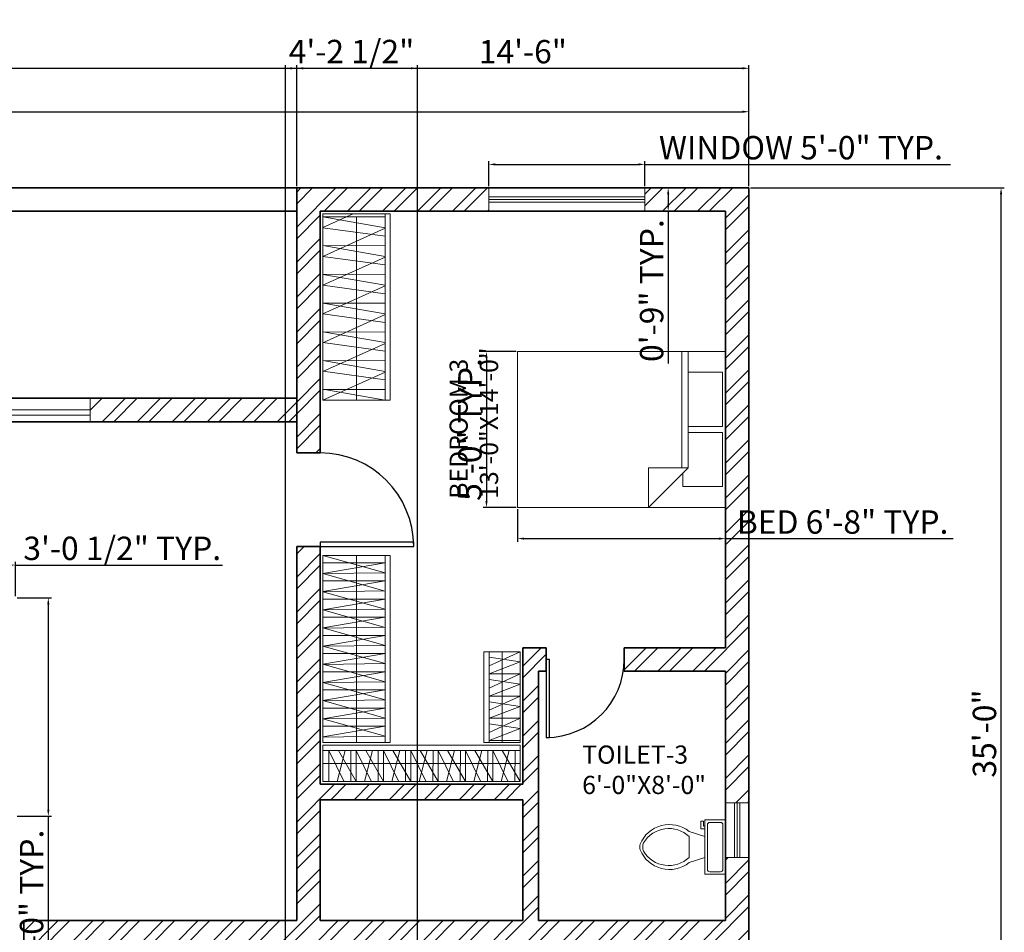
# Model space of a CAD drawing. Units: inches. Extents: x 416 to 1422, y 799 to 1634.
# Tile 5 of 5: x 1043 to 1422, y 1283 to 1634. Entities that reach past the tile are written whole.
import ezdxf

# ---------------------------------------------------------------- set-up
doc = ezdxf.new("R2010")
doc.units = ezdxf.units.IN
for name, color, linetype, lineweight in [('A-ANNO-DIMS', 2, 'Continuous', 18), ('A-AREA-IDEN', 7, 'Continuous', 18), ('A-DOOR', 4, 'Continuous', 25), ('A-FLOR-CASE', 8, 'Continuous', 18), ('A-FLOR-CASE-PATT', 252, 'Continuous', 13), ('A-FLOR-FIXT', 9, 'Continuous', 18), ('A-FURN', 8, 'Continuous', 18), ('A-GLAZ', 244, 'Continuous', 18), ('A-WALL', 7, 'Continuous', 35), ('A-WALL-PATT', 252, 'Continuous', 13)]:
    doc.layers.add(name, color=color, linetype=linetype, lineweight=lineweight)
doc.styles.get("Standard").update_dxf_attribs({"font": 'arial.ttf'})
doc.dimstyles.new('ISO-25', dxfattribs={"dimtxt": 9, "dimasz": 2.5, "dimexe": 1.25, "dimexo": 0.625, "dimtad": 1, "dimlunit": 3, "dimtxsty": 'Standard', "dimcen": 2.5, "dimadec": 0, "dimazin": 0, "dimtfac": 1, "dimtmove": 0, "dimatfit": 3, "dimfxl": 1, "dimarcsym": 0})

# ---------------------------------------------------------------- blocks, each defined once
blk = doc.blocks.new('*U4')
for p, q in [((0, 0), (0, 6)), ((40, 0), (40, 6))]:
    blk.add_line(p, q)
blk.add_lwpolyline([(0, 0), (0, -40), (1.75, -40), (1.75, 0)], close=True)
blk.add_arc((0, 0), 40, 270, 0)
blk = doc.blocks.new('*U7')
for p, q in [((9.5, -6), (9.5, -2)), ((-10, -8.5), (-8, -8.5)), ((-10, -9.5), (-10, -8.5)), ((-7, -9.5), (-10, -9.5)), ((-8, -8.5), (-8, -8)), ((-7, -8), (-7, -9.5)), ((-4, -8), (-6, -14)), ((4, -8), (6, -14)), ((4, -14), (-4, -14))]:
    blk.add_line(p, q)
blk.add_lwpolyline([(10.5, -8), (10.5, 0), (-10.5, 0), (-10.5, -8)], close=True)
for points in [[(-9.5, -2), (-9.5, -6)], [(8.5, -1), (-8.5, -1)], [(-8.5, -7), (8.5, -7)]]:
    blk.add_lwpolyline(points)
for centre, radius, start, end in [((-8.62, -1.88), 0.884, 81.8699, 188.1301), ((8.62, -1.88), 0.884, 351.8699, 98.1301), ((-8.62, -6.12), 0.884, 171.8699, 278.1301), ((8.62, -6.12), 0.884, 261.8699, 8.1301), ((3.52, -21.58), 12.17, 141.4691, 247.9714), ((4.2, -21.82), 11.33, 136.3677, 238.9468), ((-3.52, -21.58), 12.17, 292.0284, 38.5307), ((-4.2, -21.82), 11.33, 301.053, 43.6321), ((0, -27.88), 4, 245.7318, 294.2682), ((0, -29), 4, 254.8605, 285.1395)]:
    blk.add_arc(centre, radius, start, end)
blk = doc.blocks.new('Bed - Queen')
for p, q in [((0, -80.00003), (0, 0)), ((0, 0), (59.99999, 0)), ((59.99999, 0), (59.99999, -80.00003)), ((7.99999, -1.2), (28.79998, -1.2)), ((7.99999, -14.4), (7.99999, -1.2)), ((28.79998, -1.2), (28.79998, -14.4)), ((31.19999, -1.2), (51.99999, -1.2)), ((31.19999, -14.4), (31.19999, -1.2)), ((51.99999, -1.2), (51.99999, -16.4)), ((0, -14.4), (44.8, -14.4)), ((59.99999, -29.6), (44.8, -14.4)), ((44.8, -14.4), (44.8, -29.6)), ((44.8, -16.8), (0, -16.8)), ((51.99999, -16.4), (46.79936, -16.4)), ((44.8, -29.6), (59.99999, -29.6)), ((59.99999, -80.00003), (0, -80.00003))]:
    blk.add_line(p, q)
blk = doc.blocks.new('*D17')
at = {"layer": 'A-ANNO-DIMS', "color": 0, "lineweight": -2, "transparency": 16777216}
for p, q in [((483.82, 1569.64), (483.82, 1599.55)), ((1323.82, 1569.64), (1323.82, 1599.55)), ((486.32, 1598.3), (1321.32, 1598.3))]:
    blk.add_line(p, q, dxfattribs=at)
at = {"layer": 'A-ANNO-DIMS', "color": 0, "transparency": 16777216}
for points in [[(486.32, 1598.72), (486.32, 1597.88), (483.82, 1598.3)], [(1321.32, 1598.72), (1321.32, 1597.88), (1323.82, 1598.3)]]:
    blk.add_solid(points, dxfattribs=at)
at = {"layer": 'Defpoints', "color": 0, "transparency": 16777216}
for p in [(1323.82, 1598.3), (483.82, 1569.01), (1323.82, 1569.01)]:
    blk.add_point(p, dxfattribs=at)
at = {"layer": 'A-ANNO-DIMS', "color": 0, "transparency": 16777216, "insert": (903.82, 1603.52), "char_height": 9, "attachment_point": 5}
blk.add_mtext("70'", dxfattribs=at)
blk = doc.blocks.new('WIN-21IN')
for p, q in [((21, 5.5), (0, 5.5)), ((21, 4.5), (0, 4.5)), ((21, 3.5), (0, 3.5))]:
    blk.add_line(p, q)
blk.add_lwpolyline([(21, 9), (21, 0), (0, 0), (0, 9)], close=True)
blk = doc.blocks.new('WIN-60IN')
for p, q in [((3.5, 60), (3.5, 0)), ((4.5, 60), (4.5, 0)), ((5.5, 60), (5.5, 0))]:
    blk.add_line(p, q)
blk.add_lwpolyline([(0, 60), (9, 60), (9, 0), (0, 0)], close=True)
blk = doc.blocks.new('*D23')
at = {"layer": 'A-ANNO-DIMS', "color": 0, "lineweight": -2, "transparency": 16777216}
for p, q in [((1223.75, 1569.64), (1223.75, 1579.26)), ((1226.25, 1578.01), (1281.25, 1578.01)), ((1283.75, 1569.64), (1283.75, 1579.26)), ((1283.75, 1578.01), (1401.38, 1578.01))]:
    blk.add_line(p, q, dxfattribs=at)
at = {"layer": 'A-ANNO-DIMS', "color": 0, "transparency": 16777216}
for points in [[(1226.25, 1578.43), (1226.25, 1577.6), (1223.75, 1578.01)], [(1281.25, 1578.43), (1281.25, 1577.6), (1283.75, 1578.01)]]:
    blk.add_solid(points, dxfattribs=at)
at = {"layer": 'Defpoints', "color": 0, "transparency": 16777216}
for p in [(1283.75, 1578.01), (1223.75, 1569.01), (1283.75, 1569.01)]:
    blk.add_point(p, dxfattribs=at)
at = {"layer": 'A-ANNO-DIMS', "color": 0, "transparency": 16777216, "insert": (1343.82, 1583.29), "char_height": 9, "attachment_point": 5}
blk.add_mtext('WINDOW 5\'-0" TYP.', dxfattribs=at)
blk = doc.blocks.new('*D24')
at = {"layer": 'A-ANNO-DIMS', "color": 0, "lineweight": -2, "transparency": 16777216}
for p, q in [((1284.37, 1569.01), (1294, 1569.01)), ((1292.75, 1566.51), (1292.75, 1562.51)), ((1284.37, 1560.01), (1294, 1560.01)), ((1292.75, 1560.01), (1292.75, 1501.4))]:
    blk.add_line(p, q, dxfattribs=at)
at = {"layer": 'A-ANNO-DIMS', "color": 0, "transparency": 16777216}
for points in [[(1292.33, 1566.51), (1293.16, 1566.51), (1292.75, 1569.01)], [(1292.33, 1562.51), (1293.16, 1562.51), (1292.75, 1560.01)]]:
    blk.add_solid(points, dxfattribs=at)
at = {"layer": 'Defpoints', "color": 0, "transparency": 16777216}
for p in [(1283.75, 1569.01), (1283.75, 1560.01), (1292.75, 1560.01)]:
    blk.add_point(p, dxfattribs=at)
at = {"layer": 'A-ANNO-DIMS', "color": 0, "transparency": 16777216, "insert": (1287.53, 1529.46), "char_height": 9, "attachment_point": 5, "rotation": 90}
blk.add_mtext('0\'-9" TYP.', dxfattribs=at)
blk = doc.blocks.new('*D27')
at = {"layer": 'A-ANNO-DIMS', "color": 0, "lineweight": -2, "transparency": 16777216}
for p, q in [((1042.27, 1411.23), (1055.49, 1411.23)), ((1054.24, 1408.73), (1054.24, 1329.73)), ((1042.27, 1327.23), (1055.49, 1327.23)), ((1054.24, 1327.23), (1054.24, 1230.94))]:
    blk.add_line(p, q, dxfattribs=at)
at = {"layer": 'A-ANNO-DIMS', "color": 0, "transparency": 16777216}
for points in [[(1053.83, 1408.73), (1054.66, 1408.73), (1054.24, 1411.23)], [(1053.83, 1329.73), (1054.66, 1329.73), (1054.24, 1327.23)]]:
    blk.add_solid(points, dxfattribs=at)
at = {"layer": 'Defpoints', "color": 0, "transparency": 16777216}
for p in [(1041.64, 1411.23), (1041.64, 1327.23), (1054.24, 1327.23)]:
    blk.add_point(p, dxfattribs=at)
at = {"layer": 'A-ANNO-DIMS', "color": 0, "transparency": 16777216, "insert": (1048.96, 1277.83), "char_height": 9, "attachment_point": 5, "rotation": 90}
blk.add_mtext('SOFA 7\'-0" TYP.', dxfattribs=at)
blk = doc.blocks.new('*D28')
at = {"layer": 'A-ANNO-DIMS', "color": 0, "lineweight": -2, "transparency": 16777216}
for p, q in [((1004.98, 1411.86), (1004.98, 1425.08)), ((1041.64, 1411.86), (1041.64, 1425.08)), ((1007.48, 1423.83), (1039.14, 1423.83)), ((1041.64, 1423.83), (1121.22, 1423.83))]:
    blk.add_line(p, q, dxfattribs=at)
at = {"layer": 'A-ANNO-DIMS', "color": 0, "transparency": 16777216}
for points in [[(1007.48, 1424.25), (1007.48, 1423.41), (1004.98, 1423.83)], [(1039.14, 1424.25), (1039.14, 1423.41), (1041.64, 1423.83)]]:
    blk.add_solid(points, dxfattribs=at)
at = {"layer": 'Defpoints', "color": 0, "transparency": 16777216}
for p in [(1041.64, 1423.83), (1004.98, 1411.23), (1041.64, 1411.23)]:
    blk.add_point(p, dxfattribs=at)
at = {"layer": 'A-ANNO-DIMS', "color": 0, "transparency": 16777216, "insert": (1082.68, 1429.11), "char_height": 9, "attachment_point": 5}
blk.add_mtext('3\'-0 1/2" TYP.', dxfattribs=at)
blk = doc.blocks.new('*D29')
at = {"layer": 'A-ANNO-DIMS', "color": 0, "lineweight": -2, "transparency": 16777216}
for p, q in [((1234.82, 1445.39), (1234.82, 1432.76)), ((1314.82, 1445.39), (1314.82, 1432.76)), ((1237.32, 1434.01), (1312.32, 1434.01)), ((1314.82, 1434.01), (1402.38, 1434.01))]:
    blk.add_line(p, q, dxfattribs=at)
at = {"layer": 'A-ANNO-DIMS', "color": 0, "transparency": 16777216}
for points in [[(1237.32, 1434.43), (1237.32, 1433.6), (1234.82, 1434.01)], [(1312.32, 1434.43), (1312.32, 1433.6), (1314.82, 1434.01)]]:
    blk.add_solid(points, dxfattribs=at)
at = {"layer": 'Defpoints', "color": 0, "transparency": 16777216}
for p in [(1234.82, 1446.01), (1314.82, 1446.01), (1314.82, 1434.01)]:
    blk.add_point(p, dxfattribs=at)
at = {"layer": 'A-ANNO-DIMS', "color": 0, "transparency": 16777216, "insert": (1359.85, 1439.23), "char_height": 9, "attachment_point": 5}
blk.add_mtext('BED 6\'-8" TYP.', dxfattribs=at)
blk = doc.blocks.new('*D30')
at = {"layer": 'A-ANNO-DIMS', "color": 0, "lineweight": -2, "transparency": 16777216}
for p, q in [((1234.19, 1506.01), (1221.57, 1506.01)), ((1222.82, 1503.51), (1222.82, 1448.51)), ((1234.19, 1446.01), (1221.57, 1446.01))]:
    blk.add_line(p, q, dxfattribs=at)
at = {"layer": 'A-ANNO-DIMS', "color": 0, "transparency": 16777216}
for points in [[(1222.4, 1503.51), (1223.24, 1503.51), (1222.82, 1506.01)], [(1222.4, 1448.51), (1223.24, 1448.51), (1222.82, 1446.01)]]:
    blk.add_solid(points, dxfattribs=at)
at = {"layer": 'Defpoints', "color": 0, "transparency": 16777216}
for p in [(1234.82, 1506.01), (1222.82, 1446.01), (1234.82, 1446.01)]:
    blk.add_point(p, dxfattribs=at)
at = {"layer": 'A-ANNO-DIMS', "color": 0, "transparency": 16777216, "insert": (1217.6, 1476.01), "char_height": 9, "attachment_point": 5, "rotation": 90}
blk.add_mtext('5\'-0" TYP.', dxfattribs=at)
blk = doc.blocks.new('*D50')
at = {"layer": 'A-ANNO-DIMS', "color": 0, "lineweight": -2, "transparency": 16777216}
for p, q in [((1324.44, 1569.01), (1422.07, 1569.01)), ((1420.82, 1151.51), (1420.82, 1566.51)), ((1324.44, 1149.01), (1422.07, 1149.01))]:
    blk.add_line(p, q, dxfattribs=at)
at = {"layer": 'A-ANNO-DIMS', "color": 0, "transparency": 16777216}
for points in [[(1420.4, 1566.51), (1421.24, 1566.51), (1420.82, 1569.01)], [(1420.4, 1151.51), (1421.24, 1151.51), (1420.82, 1149.01)]]:
    blk.add_solid(points, dxfattribs=at)
at = {"layer": 'Defpoints', "color": 0, "transparency": 16777216}
for p in [(1323.82, 1569.01), (1420.82, 1569.01), (1323.82, 1149.01)]:
    blk.add_point(p, dxfattribs=at)
at = {"layer": 'A-ANNO-DIMS', "color": 0, "transparency": 16777216, "insert": (1415.6, 1359.01), "char_height": 9, "attachment_point": 5, "rotation": 90}
blk.add_mtext('35\'-0"', dxfattribs=at)
blk = doc.blocks.new('*D52')
at = {"layer": 'A-ANNO-DIMS', "color": 0, "lineweight": -2, "transparency": 16777216}
for p, q in [((750.82, 1569.64), (750.82, 1616.26)), ((753.32, 1615.01), (1147.32, 1615.01)), ((1149.82, 1569.64), (1149.82, 1616.26))]:
    blk.add_line(p, q, dxfattribs=at)
at = {"layer": 'A-ANNO-DIMS', "color": 0, "transparency": 16777216}
for points in [[(753.32, 1615.43), (753.32, 1614.6), (750.82, 1615.01)], [(1147.32, 1615.43), (1147.32, 1614.6), (1149.82, 1615.01)]]:
    blk.add_solid(points, dxfattribs=at)
at = {"layer": 'Defpoints', "color": 0, "transparency": 16777216}
for p in [(1149.82, 1615.01), (750.82, 1569.01), (1149.82, 1569.01)]:
    blk.add_point(p, dxfattribs=at)
at = {"layer": 'A-ANNO-DIMS', "color": 0, "transparency": 16777216, "insert": (950.32, 1620.24), "char_height": 9, "attachment_point": 5}
blk.add_mtext('33\'-3"', dxfattribs=at)
blk = doc.blocks.new('*D53')
at = {"layer": 'A-ANNO-DIMS', "color": 0, "lineweight": -2, "transparency": 16777216}
for p, q in [((1149.82, 1569.64), (1149.82, 1616.26)), ((1152.32, 1615.01), (1321.32, 1615.01)), ((1323.82, 1569.64), (1323.82, 1616.26))]:
    blk.add_line(p, q, dxfattribs=at)
at = {"layer": 'A-ANNO-DIMS', "color": 0, "transparency": 16777216}
for points in [[(1152.32, 1615.43), (1152.32, 1614.6), (1149.82, 1615.01)], [(1321.32, 1615.43), (1321.32, 1614.6), (1323.82, 1615.01)]]:
    blk.add_solid(points, dxfattribs=at)
at = {"layer": 'Defpoints', "color": 0, "transparency": 16777216}
for p in [(1323.82, 1615.01), (1149.82, 1569.01), (1323.82, 1569.01)]:
    blk.add_point(p, dxfattribs=at)
at = {"layer": 'A-ANNO-DIMS', "color": 0, "transparency": 16777216, "insert": (1236.82, 1620.23), "char_height": 9, "attachment_point": 5}
blk.add_mtext('14\'-6"', dxfattribs=at)
blk = doc.blocks.new('*D56')
at = {"layer": 'A-ANNO-DIMS', "color": 0, "lineweight": -2, "transparency": 16777216}
for p, q in [((1145.53, 1120.54), (1145.53, 1616.26)), ((1148.03, 1615.01), (1193.73, 1615.01)), ((1196.23, 1120.54), (1196.23, 1616.26))]:
    blk.add_line(p, q, dxfattribs=at)
at = {"layer": 'A-ANNO-DIMS', "color": 0, "transparency": 16777216}
for points in [[(1148.03, 1615.43), (1148.03, 1614.6), (1145.53, 1615.01)], [(1193.73, 1615.43), (1193.73, 1614.6), (1196.23, 1615.01)]]:
    blk.add_solid(points, dxfattribs=at)
at = {"layer": 'Defpoints', "color": 0, "transparency": 16777216}
for p in [(1196.23, 1615.01), (1145.53, 1119.92), (1196.23, 1119.92)]:
    blk.add_point(p, dxfattribs=at)
at = {"layer": 'A-ANNO-DIMS', "color": 0, "transparency": 16777216, "insert": (1170.88, 1620.29), "char_height": 9, "attachment_point": 5}
blk.add_mtext('4\'-2 1/2"', dxfattribs=at)

msp = doc.modelspace()

# ---------------------------------------------------------------- hatches: boundary and pattern name
at = {"layer": 'A-FLOR-CASE-PATT'}
h = msp.add_hatch(dxfattribs=at)
h.set_pattern_fill('ANSI31', color=256, scale=3.18085, angle=-20.7152, style=0)
h.paths.add_polyline_path([(1159.82, 1557.257), (1159.82, 1487.262), (1167.693, 1487.262), (1183.82, 1494.521), (1183.82, 1559.013), (1163.72, 1559.013)])
h = msp.add_hatch(dxfattribs=at)
h.set_pattern_fill('ANSI31', color=256, scale=3.48826, angle=-45.1838, style=0)
h.paths.add_polyline_path([(1159.82, 1487.858), (1183.82, 1487.858), (1183.82, 1559.013), (1159.82, 1559.013)])
h = msp.add_hatch(dxfattribs=at)
h.set_pattern_fill('ANSI31', color=256, scale=3.43151, angle=125.211, style=0)
h.paths.add_polyline_path([(1159.82, 1487.858), (1163.279, 1487.262), (1183.82, 1487.262), (1183.82, 1557.257), (1173.645, 1559.013), (1159.82, 1559.013)])
h = msp.add_hatch(dxfattribs=at)
h.set_pattern_fill('ANSI31', color=256, scale=3.44568, angle=127.257, style=0)
h.paths.add_polyline_path([(1159.82, 1557.257), (1159.82, 1494.793), (1183.82, 1491.53), (1183.82, 1553.994)])
h = msp.add_hatch(dxfattribs=at)
h.set_pattern_fill('ANSI31', color=256, scale=2.117514, angle=119.3506, style=0)
h.paths.add_polyline_path([(1159.82, 1362.45), (1183.898, 1355.705), (1183.898, 1423.068), (1167.805, 1427.576), (1159.82, 1427.576)])
h = msp.add_hatch(dxfattribs=at)
h.set_pattern_fill('ANSI31', color=256, scale=2.16963, angle=-35.3265, style=0)
h.paths.add_polyline_path([(1159.82, 1422.823), (1159.82, 1355.513), (1160.331, 1355.513), (1183.898, 1359.576), (1183.898, 1426.975)])
h = msp.add_hatch(dxfattribs=at)
h.set_pattern_fill('ANSI31', color=256, scale=2.20165, angle=-45.0628, style=0)
h.paths.add_polyline_path([(1159.82, 1426.961), (1159.82, 1359.576), (1183.898, 1359.576), (1183.898, 1426.961)])
h = msp.add_hatch(dxfattribs=at)
h.set_pattern_fill('ANSI31', color=256, scale=2.20151, angle=-44.2351, style=0)
h.paths.add_polyline_path([(1159.82, 1422.823), (1159.82, 1355.513), (1166.618, 1355.513), (1183.898, 1355.705), (1183.898, 1423.091)])
h = msp.add_hatch(dxfattribs=at)
h.set_pattern_fill('ANSI31', color=256, scale=2.45043, angle=-20.5625, style=0)
h.paths.add_polyline_path([(1223.82, 1387.782), (1223.82, 1356.693), (1235.82, 1362.128), (1235.82, 1390.484), (1229.785, 1390.484)])
h = msp.add_hatch(dxfattribs=at)
h.set_pattern_fill('ANSI31', color=256, scale=2.661494, angle=126.4514, style=0)
h.paths.add_polyline_path([(1223.82, 1359.967), (1235.82, 1358.204), (1235.82, 1389.293), (1227.712, 1390.484), (1223.82, 1390.484)])
h = msp.add_hatch(dxfattribs=at)
h.set_pattern_fill('ANSI31', color=256, scale=2.51065, angle=-24.0473, style=0)
h.paths.add_polyline_path([(1223.82, 1384.677), (1223.82, 1355.513), (1228.823, 1355.513), (1235.82, 1358.204), (1235.82, 1389.293)])
h = msp.add_hatch(dxfattribs=at)
h.set_pattern_fill('ANSI31', color=256, scale=2.69006, angle=-45.0787, style=0)
h.paths.add_polyline_path([(1223.82, 1384.677), (1223.82, 1355.513), (1235.82, 1355.513), (1235.82, 1384.677)])
h = msp.add_hatch(dxfattribs=at)
h.set_pattern_fill('ANSI31', color=256, scale=2.97981, angle=70.9408, style=0)
h.paths.add_polyline_path([(1159.82, 1350.458), (1164.703, 1340.419), (1234.55, 1340.419), (1228.667, 1352.513), (1159.82, 1352.513)])
h = msp.add_hatch(dxfattribs=at)
h.set_pattern_fill('ANSI31', color=256, scale=3.31309, angle=44.7838, style=0)
h.paths.add_polyline_path([(1159.82, 1340.513), (1228.667, 1340.513), (1228.667, 1352.513), (1159.82, 1352.513)])
h = msp.add_hatch(dxfattribs=at)
h.set_pattern_fill('ANSI31', color=256, scale=3.20716, angle=30.558, style=0)
h.paths.add_polyline_path([(1162.014, 1340.513), (1231.86, 1340.513), (1234.97, 1352.513), (1165.124, 1352.513)])
h = msp.add_hatch(dxfattribs=at)
h.set_pattern_fill('ANSI31', color=256, scale=2.86878, angle=74.9176, style=0)
h.paths.add_polyline_path([(1169.339, 1340.513), (1235.82, 1340.513), (1235.82, 1346.362), (1232.281, 1352.513), (1162.434, 1352.513)])
h = msp.add_hatch(dxfattribs=at)
h.set_pattern_fill('ANSI31', color=256, scale=3.3131, angle=44.87, style=0)
h.paths.add_polyline_path([(1167.309, 1340.513), (1235.82, 1340.513), (1235.82, 1352.513), (1167.309, 1352.513)])
at = {"layer": 'A-WALL-PATT'}
h = msp.add_hatch(dxfattribs=at)
h.set_pattern_fill('ANSI32', color=256)
h.paths.add_polyline_path([(695.32, 1569.013), (607.303, 1569.013), (607.303, 1560.013), (660.82, 1560.013), (660.82, 1419.013), (657.82, 1419.013), (657.82, 1413.013), (669.82, 1413.013), (669.82, 1446.013), (672.82, 1446.013), (672.82, 1452.013), (669.82, 1452.013), (669.82, 1560.013), (695.32, 1560.013)])
h.paths.add_polyline_path([(1323.82, 1311.283), (1314.82, 1311.283), (1314.82, 1287.013), (1242.82, 1287.013), (1242.82, 1383.013), (1245.82, 1383.013), (1245.82, 1392.013), (1236.82, 1392.013), (1236.82, 1339.513), (1158.82, 1339.513), (1158.82, 1431.013), (1149.82, 1431.013), (1149.82, 1287.013), (1044.82, 1287.013), (1044.82, 1242.013), (1053.82, 1242.013), (1053.82, 1278.013), (1221.82, 1278.013), (1221.82, 1233.013), (1230.82, 1233.013), (1230.82, 1278.013), (1314.82, 1278.013), (1314.82, 1225.894), (1323.82, 1225.894)])
h.paths.add_polyline_path([(1158.82, 1287.013), (1158.82, 1333.513), (1236.82, 1333.513), (1236.82, 1287.013)], flags=16)
h.paths.add_polyline_path([(1323.82, 1569.013), (1283.747, 1569.013), (1283.747, 1560.013), (1314.82, 1560.013), (1314.82, 1392.013), (1275.82, 1392.013), (1275.82, 1383.013), (1314.82, 1383.013), (1314.82, 1332.283), (1323.82, 1332.283)])
h.paths.add_polyline_path([(750.82, 1569.013), (716.32, 1569.013), (716.32, 1560.013), (741.82, 1560.013), (741.82, 1452.013), (702.82, 1452.013), (702.82, 1447.513), (702.82, 1446.013), (741.82, 1446.013), (741.82, 1287.013), (750.82, 1287.013)])
h.paths.add_polyline_path([(1158.82, 1560.013), (1223.747, 1560.013), (1223.747, 1569.013), (1149.82, 1569.013), (1149.82, 1467.013), (1158.82, 1467.013)])
h.paths.add_polyline_path([(1323.82, 1098.013), (1230.82, 1098.013), (1230.82, 1149.013), (1323.82, 1149.013), (1323.82, 1204.894), (1314.82, 1204.894), (1314.82, 1158.013), (1230.82, 1158.013), (1230.82, 1203.013), (1221.82, 1203.013), (1221.82, 1098.013), (1053.82, 1098.013), (1053.82, 1194.013), (1044.82, 1194.013), (1044.82, 1089.013), (1104.82, 1089.013), (1104.82, 1086.013), (1113.82, 1086.013), (1113.82, 1089.013), (1194.82, 1089.013), (1314.82, 1089.013), (1314.82, 897.013), (1194.82, 897.013), (1194.82, 1041.013), (1113.82, 1041.013), (1113.82, 1044.013), (1104.82, 1044.013), (1104.82, 1032.013), (1113.82, 1032.013), (1113.82, 1035.013), (1185.82, 1035.013), (1185.82, 969.013), (1113.82, 969.013), (1113.82, 1008.013), (1104.82, 1008.013), (1104.82, 969.013), (1088.452, 969.013), (1088.452, 960.013), (1185.82, 960.013), (1185.82, 888.013), (1323.82, 888.013)])
h = msp.add_hatch(dxfattribs=at)
h.set_pattern_fill('ANSI32', color=256)
h.paths.add_polyline_path([(830.32, 1488.013), (750.82, 1488.013), (750.82, 1479.013), (830.32, 1479.013)])
h.paths.add_polyline_path([(1149.82, 1488.013), (1070.32, 1488.013), (1070.32, 1479.013), (1149.82, 1479.013)])

# ---------------------------------------------------------------- linework, layer by layer
at = {"layer": 'A-FLOR-CASE'}
for p, q in [((1159.82, 1487.262), (1159.82, 1559.013)), ((1159.82, 1559.013), (1185.82, 1559.013)), ((1172.82, 1557.854), (1172.82, 1487.262)), ((1183.82, 1487.262), (1183.82, 1559.013)), ((1185.82, 1487.262), (1185.82, 1559.013)), ((1159.82, 1487.262), (1185.82, 1487.262)), ((1159.82, 1427.576), (1185.82, 1427.576)), ((1159.82, 1355.513), (1159.82, 1427.576)), ((1172.82, 1355.513), (1172.82, 1427.576)), ((1183.82, 1355.513), (1183.82, 1427.576)), ((1185.82, 1355.513), (1185.82, 1427.576)), ((1221.82, 1355.513), (1221.82, 1390.484)), ((1235.82, 1390.484), (1221.82, 1390.484)), ((1223.82, 1355.513), (1223.82, 1390.484)), ((1228.82, 1355.513), (1228.82, 1390.484)), ((1235.82, 1355.513), (1235.82, 1390.484)), ((1185.82, 1355.513), (1159.82, 1355.513)), ((1159.82, 1340.513), (1159.82, 1354.513)), ((1235.82, 1354.513), (1159.82, 1354.513)), ((1235.82, 1352.513), (1159.82, 1352.513)), ((1235.82, 1355.513), (1221.82, 1355.513)), ((1235.82, 1340.513), (1235.82, 1354.513)), ((1159.82, 1347.513), (1235.82, 1347.513)), ((1235.82, 1340.513), (1159.82, 1340.513))]:
    msp.add_line(p, q, dxfattribs=at)
at = {"layer": 'A-FLOR-CASE-PATT'}
for p, q in [((1235.82, 1386.56), (1235.82, 1386.56)), ((1223.82, 1381.943), (1223.82, 1381.943))]:
    msp.add_line(p, q, dxfattribs=at)
at = {"layer": 'A-GLAZ'}
for p, q in [((1070.32, 1479.013), (1070.32, 1488.013)), ((830.32, 1483.513), (1070.32, 1483.513)), ((878.32, 1481.513), (1070.32, 1481.513))]:
    msp.add_line(p, q, dxfattribs=at)
at = {"layer": 'A-WALL'}
for p, q in [((483.82, 1569.013), (1323.82, 1569.013)), ((1149.82, 1467.013), (1149.82, 1569.013)), ((1323.82, 1569.013), (1323.82, 1149.013)), ((750.82, 1560.013), (1149.82, 1560.013)), ((1158.82, 1467.013), (1158.82, 1560.013)), ((1158.82, 1560.013), (1314.82, 1560.013)), ((1314.82, 1392.013), (1314.82, 1560.013)), ((750.82, 1488.013), (1149.82, 1488.013)), ((750.82, 1479.013), (1149.82, 1479.013)), ((1149.82, 1467.013), (1158.82, 1467.013)), ((1149.82, 1287.013), (1149.82, 1431.013)), ((1149.82, 1431.013), (1158.82, 1431.013)), ((1158.82, 1339.513), (1158.82, 1431.013)), ((1236.82, 1392.013), (1245.82, 1392.013)), ((1236.82, 1339.513), (1236.82, 1392.013)), ((1245.82, 1383.013), (1245.82, 1392.013)), ((1275.82, 1383.013), (1275.82, 1392.013)), ((1275.82, 1392.013), (1314.82, 1392.013)), ((1242.82, 1287.013), (1242.82, 1383.013)), ((1242.82, 1383.013), (1245.82, 1383.013)), ((1275.82, 1383.013), (1314.82, 1383.013)), ((1314.82, 1287.013), (1314.82, 1383.013)), ((1236.82, 1339.513), (1158.82, 1339.513)), ((1158.82, 1287.013), (1158.82, 1333.513)), ((1236.82, 1333.513), (1158.82, 1333.513)), ((1236.82, 1287.013), (1236.82, 1333.513)), ((1044.82, 1287.013), (1149.82, 1287.013)), ((1044.82, 1242.013), (1044.82, 1287.013)), ((1158.82, 1287.013), (1236.82, 1287.013)), ((1242.82, 1287.013), (1314.82, 1287.013))]:
    msp.add_line(p, q, dxfattribs=at)

# ---------------------------------------------------------------- block references
at = {"layer": 'A-DOOR', "xscale": 0.8999999999999942, "yscale": 0.8999999999999942, "zscale": 0.8999999999999942, "rotation": 89.99999999999994}
msp.add_blockref('*U4', (1158.82, 1431.013), dxfattribs=at)
at = {"layer": 'A-DOOR', "xscale": 0.75, "yscale": 0.75, "zscale": 0.75}
msp.add_blockref('*U4', (1245.82, 1387.513), dxfattribs=at)
at = {"layer": 'A-FLOR-FIXT', "rotation": 270}
msp.add_blockref('*U7', (1314.82, 1315.333), dxfattribs=at)
at = {"layer": 'A-FURN', "rotation": 270}
msp.add_blockref('Bed - Queen', (1314.82, 1506.013), dxfattribs=at)
at = {"layer": 'A-GLAZ'}
for name, p, rotation in [('WIN-60IN', (1223.747, 1569.012), 270.0000000000007), ('WIN-21IN', (1323.819, 1311.283), 89.9999999999983)]:
    msp.add_blockref(name, p, dxfattribs=dict(at, rotation=rotation))

# ---------------------------------------------------------------- texts
at = {"layer": 'A-AREA-IDEN', "insert": (1208.635, 1449.331), "char_height": 7, "attachment_point": 1, "rotation": 90}
msp.add_mtext_dynamic_manual_height_columns('BEDROOM 3\\P13\'-0"X14\'-0"', width=62.77808, gutter_width=12.5, heights=[0], dxfattribs=at)
at = {"layer": 'A-AREA-IDEN', "insert": (1259.65, 1354.396), "char_height": 7, "attachment_point": 1}
msp.add_mtext_dynamic_manual_height_columns('TOILET-3 \\P6\'-0"X8\'-0"', width=44.45572, gutter_width=12.5, heights=[0], dxfattribs=at)

# ---------------------------------------------------------------- dimensions: what is measured, and where the dimension line sits
at = {"layer": 'A-ANNO-DIMS'}
for base, p1, p2, override, picture, middle in [((1196.227, 1615.013), (1145.527, 1119.918), (1196.227, 1119.918), {"dimdec": 1, "dimlfac": 1, "dimrnd": 0, "dimzin": 1, "dimdsep": 46, "dimlunit": 4, "dimfrac": 2}, '*D56', (1170.877, 1620.291)), ((1149.82, 1615.013), (750.82, 1569.013), (1149.82, 1569.013), {"dimdec": 1, "dimlfac": 1, "dimrnd": 0, "dimzin": 1, "dimdsep": 46, "dimlunit": 4, "dimfrac": 2}, '*D52', (950.32, 1620.236)), ((1323.82, 1615.013), (1149.82, 1569.013), (1323.82, 1569.013), {"dimdec": 1, "dimlfac": 1, "dimrnd": 0, "dimzin": 1, "dimdsep": 46, "dimlunit": 4, "dimfrac": 2}, '*D53', (1236.82, 1620.233)), ((1323.82, 1598.301), (483.82, 1569.013), (1323.82, 1569.013), {"dimclrd": 0, "dimclre": 0, "dimclrt": 0}, '*D17', (903.82, 1603.522))]:
    dim = msp.add_linear_dim(base=base, p1=p1, p2=p2, dimstyle='ISO-25', override=override, dxfattribs=at)
    dim.commit()
    dim.dimension.update_dxf_attribs({"geometry": picture, "text_midpoint": middle})
for base, p1, p2, angle, text, picture, middle in [((1283.747, 1578.013), (1223.747, 1569.013), (1283.747, 1569.013), 0, 'WINDOW <> TYP.', '*D23', (1343.815, 1583.294)), ((1292.747, 1560.013), (1283.747, 1569.013), (1283.747, 1560.013), 270, '<> TYP.', '*D24', (1287.527, 1529.458)), ((1222.82, 1446.013), (1234.82, 1506.013), (1234.82, 1446.013), 270, '<> TYP.', '*D30', (1217.6, 1476.013)), ((1054.243, 1327.231), (1041.643, 1411.231), (1041.643, 1327.231), 270, 'SOFA <> TYP.', '*D27', (1048.961, 1277.835))]:
    dim = msp.add_linear_dim(base=base, p1=p1, p2=p2, angle=angle, text=text, dimstyle='ISO-25', override={"dimdec": 1, "dimlfac": 1, "dimrnd": 0, "dimzin": 1, "dimdsep": 46, "dimlunit": 4, "dimfrac": 2}, dxfattribs=at)
    dim.commit()
    dim.dimension.update_dxf_attribs({"geometry": picture, "text_midpoint": middle})
dim = msp.add_linear_dim(base=(1420.82, 1569.013), p1=(1323.82, 1149.013), p2=(1323.82, 1569.013), angle=90, dimstyle='ISO-25', override={"dimdec": 1, "dimlfac": 1, "dimrnd": 0, "dimzin": 1, "dimdsep": 46, "dimlunit": 4, "dimfrac": 2}, dxfattribs=at)
dim.commit()
dim.dimension.update_dxf_attribs({"geometry": '*D50', "text_midpoint": (1415.597, 1359.013)})
for base, p1, p2, text, picture, middle in [((1314.82, 1434.013), (1234.82, 1446.013), (1314.82, 1446.013), 'BED <> TYP.', '*D29', (1359.848, 1439.233)), ((1041.643, 1423.831), (1004.976, 1411.231), (1041.643, 1411.231), '<> TYP.', '*D28', (1082.68, 1429.112))]:
    dim = msp.add_linear_dim(base=base, p1=p1, p2=p2, text=text, dimstyle='ISO-25', override={"dimdec": 1, "dimlfac": 1, "dimrnd": 0, "dimzin": 1, "dimdsep": 46, "dimlunit": 4, "dimfrac": 2}, dxfattribs=at)
    dim.commit()
    dim.dimension.update_dxf_attribs({"geometry": picture, "text_midpoint": middle})

doc.saveas('drawing.dxf')
